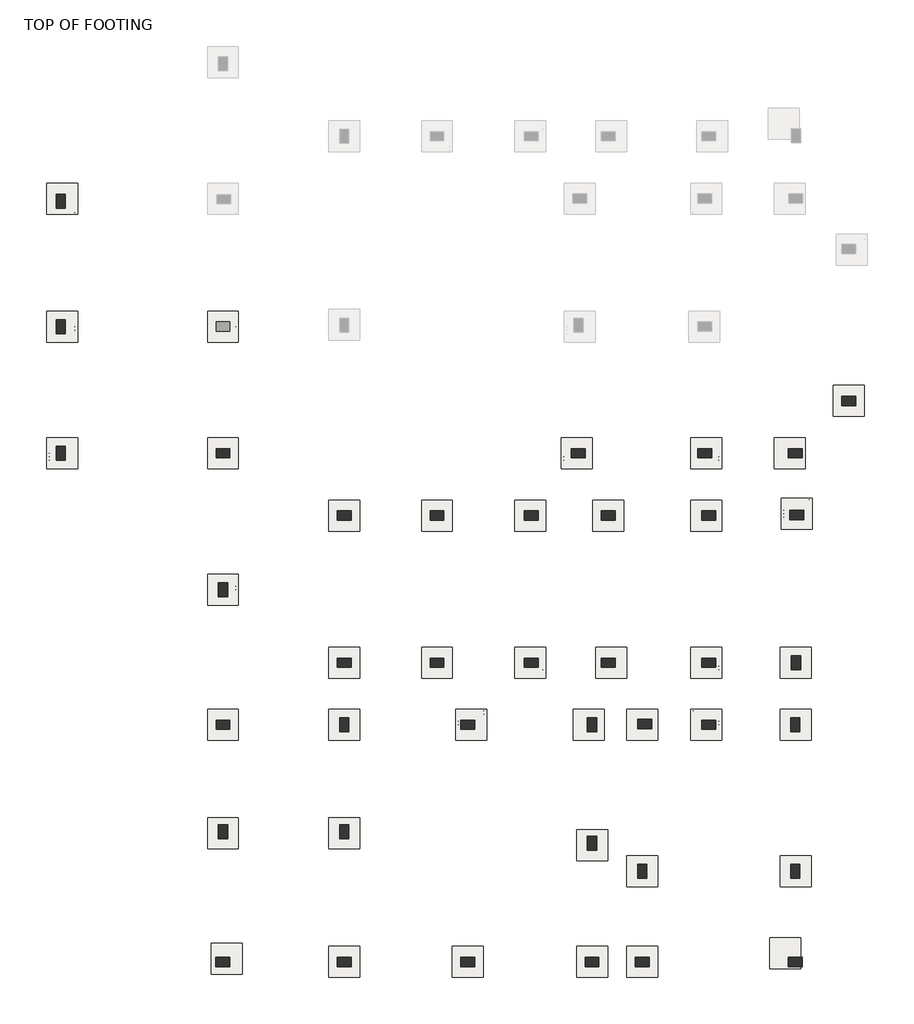
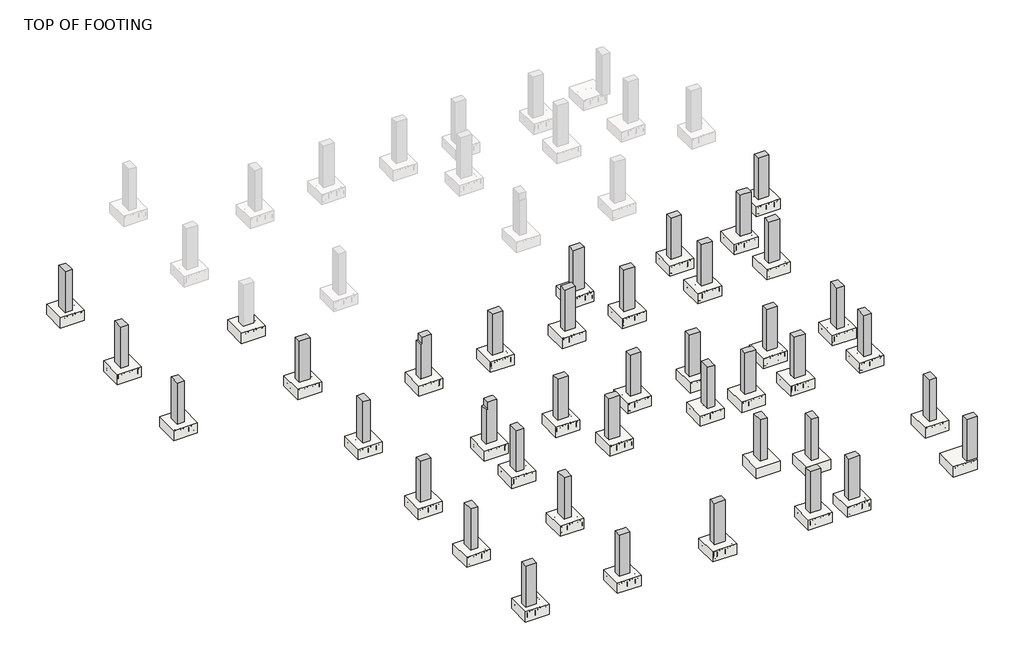
# One storey, part 1 of 20: 40 slabs, 39 columns.
"""IFC4 building model written with IfcOpenShell, lengths in millimetres."""

from ifc_helpers import new_model, si_unit, origin, place, context, project, spatial, faceted_brep, transform, mapped, element, save
from components import m_footing_rectangular_4c97ae35

model = new_model("IFC4")

# Units and contexts
model_context = context("Model", 3, world=origin())
ifc_project = project(units=[si_unit("LENGTHUNIT", "METRE", prefix="MILLI")], contexts=[model_context])

# Site, building, storey
site = spatial("IfcSite", under=ifc_project)
building = spatial("IfcBuilding", under=site)
storey = spatial("IfcBuildingStorey", under=building, Name="TOP OF FOOTING", Elevation=-1828.8)

# Columns
placement = place(None, origin())
element("IfcColumn", 1, ObjectType="M_Concrete-Rectangular-Column : 300 x 450mm", at=placement, inside=storey, context=model_context, shape_type="Brep", body=[
    faceted_brep([(-10828.8105653, 5382.6057249, -1828.8), (-10828.8105653, 4932.6057249, -1828.8), (-11128.8105653, 4932.6057249, -1828.8), (-11128.8105653, 5382.6057249, -1828.8), (-10828.8105653, 5382.6057249, 0.0), (-10828.8105653, 5067.6057249, 0.0), (-10828.8105653, 4932.6057249, 0.0), (-11128.8105653, 4932.6057249, 0.0), (-11128.8105653, 5382.6057249, 0.0)], [[[0, 1, 2, 3]], [[4, 5, 6, 1, 0]], [[6, 7, 2, 1]], [[7, 8, 3, 2]], [[8, 4, 0, 3]], [[4, 8, 7, 6, 5]]]),
])
element("IfcColumn", 2, ObjectType="M_Concrete-Rectangular-Column : 300 x 450mm", at=placement, inside=storey, context=model_context, shape_type="Brep", body=[
    faceted_brep([(-11128.8105653, 876.1713929, -1828.8), (-11128.8105653, 1326.1713929, -1828.8), (-10828.8105653, 1326.1713929, -1828.8), (-10828.8105653, 876.1713929, -1828.8), (-11128.8105653, 876.1713929, 0.0), (-11128.8105653, 1326.1713929, 0.0), (-10828.8105653, 1326.1713929, 0.0), (-10828.8105653, 1251.1713929, 0.0), (-10828.8105653, 951.1713929, 0.0), (-10828.8105653, 876.1713929, 0.0)], [[[0, 1, 2, 3]], [[4, 5, 1, 0]], [[5, 6, 2, 1]], [[6, 7, 8, 9, 3, 2]], [[9, 4, 0, 3]], [[4, 9, 8, 7, 6, 5]]]),
])
element("IfcColumn", 3, ObjectType="M_Concrete-Rectangular-Column : 300 x 450mm", at=placement, inside=storey, context=model_context, shape_type="Brep", body=[
    faceted_brep([(14244.1163908, -1148.8286071, -1828.8), (14694.1163908, -1148.8286071, -1828.8), (14694.1163908, -1448.8286071, -1828.8), (14244.1163908, -1448.8286071, -1828.8), (14244.1163908, -1148.8286071, -300.0), (14244.1163908, -1148.8286071, 0.0), (14319.1163908, -1148.8286071, 0.0), (14694.1163908, -1148.8286071, 0.0), (14694.1163908, -1448.8286071, 0.0), (14244.1163908, -1448.8286071, 0.0)], [[[0, 1, 2, 3]], [[1, 0, 4, 5, 6, 7]], [[2, 1, 7, 8]], [[3, 2, 8, 9]], [[0, 3, 9, 5, 4]], [[8, 7, 6, 5, 9]]]),
])
element("IfcColumn", 4, ObjectType="M_Concrete-Rectangular-Column : 300 x 450mm", at=placement, inside=storey, context=model_context, shape_type="Brep", body=[
    faceted_brep([(12524.1163908, -2839.4535766, -1828.8), (12974.1163908, -2839.4535766, -1828.8), (12974.1163908, -3139.4535766, -1828.8), (12524.1163908, -3139.4535766, -1828.8), (12524.1163908, -2839.4535766, -300.0), (12524.1163908, -2839.4535766, 0.0), (12599.1163908, -2839.4535766, 0.0), (12974.1163908, -2839.4535766, 0.0), (12974.1163908, -3139.4535766, 0.0), (12619.1163908, -3139.4535766, 0.0), (12524.1163908, -3139.4535766, 0.0), (12524.1163908, -3139.4535766, -300.0)], [[[0, 1, 2, 3]], [[1, 0, 4, 5, 6, 7]], [[2, 1, 7, 8]], [[3, 2, 8, 9, 10, 11]], [[0, 3, 11, 10, 5, 4]], [[8, 7, 6, 5, 10, 9]]]),
])
element("IfcColumn", 5, ObjectType="M_Concrete-Rectangular-Column : 300 x 450mm", at=placement, inside=storey, context=model_context, shape_type="Brep", body=[
    faceted_brep([(9601.8679014, -2839.4535766, -1828.8), (10051.8679014, -2839.4535766, -1828.8), (10051.8679014, -3139.4535766, -1828.8), (9601.8679014, -3139.4535766, -1828.8), (9601.8679014, -2839.4535766, -300.0), (9601.8679014, -2839.4535766, 0.0), (10051.8679014, -2839.4535766, 0.0), (10051.8679014, -2839.4535766, -300.0), (10051.8679014, -3139.4535766, 0.0), (10051.8679014, -3139.4535766, -300.0), (9601.8679014, -3139.4535766, 0.0), (9601.8679014, -3139.4535766, -300.0)], [[[0, 1, 2, 3]], [[1, 0, 4, 5, 6, 7]], [[2, 1, 7, 6, 8, 9]], [[3, 2, 9, 8, 10, 11]], [[0, 3, 11, 10, 5, 4]], [[6, 5, 10, 8]]]),
])
element("IfcColumn", 6, ObjectType="M_Concrete-Rectangular-Column : 300 x 450mm", at=placement, inside=storey, context=model_context, shape_type="Brep", body=[
    faceted_brep([(5517.5248054, -2839.4535766, -1828.8), (5967.5248054, -2839.4535766, -1828.8), (5967.5248054, -3139.4535766, -1828.8), (5517.5248054, -3139.4535766, -1828.8), (5517.5248054, -2839.4535766, -300.0), (5517.5248054, -2839.4535766, 0.0), (5967.5248054, -2839.4535766, 0.0), (5967.5248054, -2839.4535766, -300.0), (5967.5248054, -3139.4535766, 0.0), (5967.5248054, -3139.4535766, -300.0), (5517.5248054, -3139.4535766, 0.0), (5517.5248054, -3139.4535766, -300.0)], [[[0, 1, 2, 3]], [[1, 0, 4, 5, 6, 7]], [[2, 1, 7, 6, 8, 9]], [[3, 2, 9, 8, 10, 11]], [[0, 3, 11, 10, 5, 4]], [[6, 5, 10, 8]]]),
])
element("IfcColumn", 7, ObjectType="M_Concrete-Rectangular-Column : 300 x 450mm", at=placement, inside=storey, context=model_context, shape_type="Brep", body=[
    faceted_brep([(-11128.8105653, -3214.4535766, -1828.8), (-11128.8105653, -2764.4535766, -1828.8), (-10828.8105653, -2764.4535766, -1828.8), (-10828.8105653, -3214.4535766, -1828.8), (-11128.8105653, -3214.4535766, 0.0), (-11128.8105653, -2764.4535766, 0.0), (-10828.8105653, -2764.4535766, 0.0), (-10828.8105653, -2839.4535766, 0.0), (-10828.8105653, -3214.4535766, 0.0)], [[[0, 1, 2, 3]], [[4, 5, 1, 0]], [[5, 6, 2, 1]], [[6, 7, 8, 3, 2]], [[8, 4, 0, 3]], [[4, 8, 7, 6, 5]]]),
])
element("IfcColumn", 8, ObjectType="M_Concrete-Rectangular-Column : 300 x 450mm", at=placement, inside=storey, context=model_context, shape_type="Brep", body=[
    faceted_brep([(-5513.8105653, -3139.4535766, -1828.8), (-5963.8105653, -3139.4535766, -1828.8), (-5963.8105653, -2839.4535766, -1828.8), (-5513.8105653, -2839.4535766, -1828.8), (-5513.8105653, -3139.4535766, -300.0), (-5513.8105653, -3139.4535766, 0.0), (-5588.8105653, -3139.4535766, 0.0), (-5963.8105653, -3139.4535766, 0.0), (-5963.8105653, -2839.4535766, 0.0), (-5963.8105653, -2839.4535766, -300.0), (-5513.8105653, -2839.4535766, 0.0), (-5513.8105653, -2839.4535766, -300.0)], [[[0, 1, 2, 3]], [[1, 0, 4, 5, 6, 7]], [[2, 1, 7, 8, 9]], [[3, 2, 9, 8, 10, 11]], [[0, 3, 11, 10, 5, 4]], [[8, 7, 6, 5, 10]]]),
])
element("IfcColumn", 9, ObjectType="M_Concrete-Rectangular-Column : 300 x 450mm", at=placement, inside=storey, context=model_context, shape_type="Brep", body=[
    faceted_brep([(-1596.7865686, -5151.6229916, -1828.8), (-2046.7865686, -5151.6229916, -1828.8), (-2046.7865686, -4851.6229916, -1828.8), (-1596.7865686, -4851.6229916, -1828.8), (-1596.7865686, -5151.6229916, -300.0), (-1596.7865686, -5151.6229916, 0.0), (-1671.7865686, -5151.6229916, 0.0), (-1971.7865686, -5151.6229916, 0.0), (-1971.7865686, -5151.6229916, -300.0), (-2046.7865686, -5151.6229916, -300.0), (-2046.7865686, -4851.6229916, -300.0), (-1971.7865686, -4851.6229916, -300.0), (-1971.7865686, -4851.6229916, 0.0), (-1671.7865686, -4851.6229916, 0.0), (-1596.7865686, -4851.6229916, 0.0), (-1596.7865686, -4851.6229916, -300.0)], [[[0, 1, 2, 3]], [[1, 0, 4, 5, 6, 7, 8, 9]], [[2, 1, 9, 10]], [[3, 2, 10, 11, 12, 13, 14, 15]], [[0, 3, 15, 14, 5, 4]], [[5, 14, 13, 12, 7, 6]], [[8, 11, 10, 9]], [[11, 8, 7, 12]]]),
])
element("IfcColumn", 10, ObjectType="M_Concrete-Rectangular-Column : 300 x 450mm", at=placement, inside=storey, context=model_context, shape_type="Brep", body=[
    faceted_brep([(1399.7296816, -5151.6229916, -1828.8), (949.7296816, -5151.6229916, -1828.8), (949.7296816, -4851.6229916, -1828.8), (1399.7296816, -4851.6229916, -1828.8), (1399.7296816, -5151.6229916, -300.0), (1399.7296816, -5151.6229916, 0.0), (949.7296816, -5151.6229916, 0.0), (949.7296816, -5151.6229916, -300.0), (949.7296816, -4851.6229916, 0.0), (949.7296816, -4851.6229916, -300.0), (1399.7296816, -4851.6229916, 0.0), (1399.7296816, -4851.6229916, -300.0)], [[[0, 1, 2, 3]], [[1, 0, 4, 5, 6, 7]], [[2, 1, 7, 6, 8, 9]], [[3, 2, 9, 8, 10, 11]], [[0, 3, 11, 10, 5, 4]], [[6, 5, 10, 8]]]),
])
element("IfcColumn", 11, ObjectType="M_Concrete-Rectangular-Column : 300 x 450mm", at=placement, inside=storey, context=model_context, shape_type="Brep", body=[
    faceted_brep([(4447.5248054, -5151.6229916, -1828.8), (3997.5248054, -5151.6229916, -1828.8), (3997.5248054, -4851.6229916, -1828.8), (4447.5248054, -4851.6229916, -1828.8), (4447.5248054, -5151.6229916, -300.0), (4447.5248054, -5151.6229916, 0.0), (3997.5248054, -5151.6229916, 0.0), (3997.5248054, -5151.6229916, -300.0), (3997.5248054, -4851.6229916, 0.0), (3997.5248054, -4851.6229916, -300.0), (4447.5248054, -4851.6229916, 0.0), (4447.5248054, -4851.6229916, -300.0)], [[[0, 1, 2, 3]], [[1, 0, 4, 5, 6, 7]], [[2, 1, 7, 6, 8, 9]], [[3, 2, 9, 8, 10, 11]], [[0, 3, 11, 10, 5, 4]], [[6, 5, 10, 8]]]),
])
element("IfcColumn", 12, ObjectType="M_Concrete-Rectangular-Column : 300 x 450mm", at=placement, inside=storey, context=model_context, shape_type="Brep", body=[
    faceted_brep([(6931.8679014, -5151.6229916, -1828.8), (6481.8679014, -5151.6229916, -1828.8), (6481.8679014, -4851.6229916, -1828.8), (6931.8679014, -4851.6229916, -1828.8), (6931.8679014, -5151.6229916, -300.0), (6931.8679014, -5151.6229916, 0.0), (6481.8679014, -5151.6229916, 0.0), (6481.8679014, -5151.6229916, -300.0), (6481.8679014, -4851.6229916, 0.0), (6931.8679014, -4851.6229916, 0.0)], [[[0, 1, 2, 3]], [[1, 0, 4, 5, 6, 7]], [[2, 1, 7, 6, 8]], [[3, 2, 8, 9]], [[0, 3, 9, 5, 4]], [[6, 5, 9, 8]]]),
])
element("IfcColumn", 13, ObjectType="M_Concrete-Rectangular-Column : 300 x 450mm", at=placement, inside=storey, context=model_context, shape_type="Brep", body=[
    faceted_brep([(10171.8679014, -5151.6229916, -1828.8), (9721.8679014, -5151.6229916, -1828.8), (9721.8679014, -4851.6229916, -1828.8), (10171.8679014, -4851.6229916, -1828.8), (10171.8679014, -5151.6229916, -300.0), (10171.8679014, -5151.6229916, 0.0), (9721.8679014, -5151.6229916, 0.0), (9721.8679014, -5151.6229916, -300.0), (9721.8679014, -4851.6229916, 0.0), (10171.8679014, -4851.6229916, 0.0)], [[[0, 1, 2, 3]], [[1, 0, 4, 5, 6, 7]], [[2, 1, 7, 6, 8]], [[3, 2, 8, 9]], [[0, 3, 9, 5, 4]], [[6, 5, 9, 8]]]),
])
element("IfcColumn", 14, ObjectType="M_Concrete-Rectangular-Column : 300 x 450mm", at=placement, inside=storey, context=model_context, shape_type="Brep", body=[
    faceted_brep([(13014.1163908, -5131.6229916, -1828.8), (12564.1163908, -5131.6229916, -1828.8), (12564.1163908, -4831.6229916, -1828.8), (13014.1163908, -4831.6229916, -1828.8), (13014.1163908, -5131.6229916, 0.0), (12564.1163908, -5131.6229916, 0.0), (12564.1163908, -4831.6229916, 0.0), (12564.1163908, -4831.6229916, -300.0), (12619.1163908, -4831.6229916, 0.0), (13014.1163908, -4831.6229916, 0.0)], [[[0, 1, 2, 3]], [[1, 0, 4, 5]], [[2, 1, 5, 6, 7]], [[3, 2, 7, 6, 8, 9]], [[0, 3, 9, 4]], [[5, 4, 9, 8, 6]]]),
])
element("IfcColumn", 15, ObjectType="M_Concrete-Rectangular-Column : 300 x 450mm", at=placement, inside=storey, context=model_context, shape_type="Brep", body=[
    faceted_brep([(-1596.7865686, -9907.1078267, -1828.8), (-2046.7865686, -9907.1078267, -1828.8), (-2046.7865686, -9607.1078267, -1828.8), (-1596.7865686, -9607.1078267, -1828.8), (-1596.7865686, -9907.1078267, -300.0), (-1596.7865686, -9907.1078267, 0.0), (-1671.7865686, -9907.1078267, 0.0), (-1971.7865686, -9907.1078267, 0.0), (-1971.7865686, -9907.1078267, -300.0), (-2046.7865686, -9907.1078267, -300.0), (-2046.7865686, -9607.1078267, -300.0), (-1971.7865686, -9607.1078267, -300.0), (-1971.7865686, -9607.1078267, 0.0), (-1671.7865686, -9607.1078267, 0.0), (-1596.7865686, -9607.1078267, 0.0), (-1596.7865686, -9607.1078267, -300.0)], [[[0, 1, 2, 3]], [[1, 0, 4, 5, 6, 7, 8, 9]], [[2, 1, 9, 10]], [[3, 2, 10, 11, 12, 13, 14, 15]], [[0, 3, 15, 14, 5, 4]], [[5, 14, 13, 12, 7, 6]], [[8, 11, 10, 9]], [[11, 8, 7, 12]]]),
])
element("IfcColumn", 16, ObjectType="M_Concrete-Rectangular-Column : 300 x 450mm", at=placement, inside=storey, context=model_context, shape_type="Brep", body=[
    faceted_brep([(1399.7296816, -9907.1078267, -1828.8), (949.7296816, -9907.1078267, -1828.8), (949.7296816, -9607.1078267, -1828.8), (1399.7296816, -9607.1078267, -1828.8), (1399.7296816, -9907.1078267, -300.0), (1399.7296816, -9907.1078267, 0.0), (949.7296816, -9907.1078267, 0.0), (949.7296816, -9907.1078267, -300.0), (949.7296816, -9607.1078267, 0.0), (949.7296816, -9607.1078267, -300.0), (1399.7296816, -9607.1078267, 0.0), (1399.7296816, -9607.1078267, -300.0)], [[[0, 1, 2, 3]], [[1, 0, 4, 5, 6, 7]], [[2, 1, 7, 6, 8, 9]], [[3, 2, 9, 8, 10, 11]], [[0, 3, 11, 10, 5, 4]], [[6, 5, 10, 8]]]),
])
element("IfcColumn", 17, ObjectType="M_Concrete-Rectangular-Column : 300 x 450mm", at=placement, inside=storey, context=model_context, shape_type="Brep", body=[
    faceted_brep([(4447.5248054, -9907.1078267, -1828.8), (3997.5248054, -9907.1078267, -1828.8), (3997.5248054, -9607.1078267, -1828.8), (4447.5248054, -9607.1078267, -1828.8), (4447.5248054, -9907.1078267, -300.0), (4447.5248054, -9907.1078267, 0.0), (3997.5248054, -9907.1078267, 0.0), (3997.5248054, -9907.1078267, -300.0), (3997.5248054, -9607.1078267, 0.0), (3997.5248054, -9607.1078267, -300.0), (4447.5248054, -9607.1078267, 0.0), (4447.5248054, -9607.1078267, -300.0)], [[[0, 1, 2, 3]], [[1, 0, 4, 5, 6, 7]], [[2, 1, 7, 6, 8, 9]], [[3, 2, 9, 8, 10, 11]], [[0, 3, 11, 10, 5, 4]], [[6, 5, 10, 8]]]),
])
element("IfcColumn", 18, ObjectType="M_Concrete-Rectangular-Column : 300 x 450mm", at=placement, inside=storey, context=model_context, shape_type="Brep", body=[
    faceted_brep([(6931.8679014, -9907.1078267, -1828.8), (6481.8679014, -9907.1078267, -1828.8), (6481.8679014, -9607.1078267, -1828.8), (6931.8679014, -9607.1078267, -1828.8), (6931.8679014, -9907.1078267, -300.0), (6931.8679014, -9907.1078267, 0.0), (6481.8679014, -9907.1078267, 0.0), (6481.8679014, -9907.1078267, -300.0), (6481.8679014, -9607.1078267, 0.0), (6481.8679014, -9607.1078267, -300.0), (6931.8679014, -9607.1078267, 0.0), (6931.8679014, -9607.1078267, -300.0)], [[[0, 1, 2, 3]], [[1, 0, 4, 5, 6, 7]], [[2, 1, 7, 6, 8, 9]], [[3, 2, 9, 8, 10, 11]], [[0, 3, 11, 10, 5, 4]], [[6, 5, 10, 8]]]),
])
element("IfcColumn", 19, ObjectType="M_Concrete-Rectangular-Column : 300 x 450mm", at=placement, inside=storey, context=model_context, shape_type="Brep", body=[
    faceted_brep([(10171.8679014, -9907.1078267, -1828.8), (9721.8679014, -9907.1078267, -1828.8), (9721.8679014, -9607.1078267, -1828.8), (10171.8679014, -9607.1078267, -1828.8), (10171.8679014, -9907.1078267, -300.0), (10171.8679014, -9907.1078267, 0.0), (9721.8679014, -9907.1078267, 0.0), (9721.8679014, -9907.1078267, -300.0), (9721.8679014, -9607.1078267, 0.0), (9721.8679014, -9607.1078267, -300.0), (10171.8679014, -9607.1078267, 0.0), (10171.8679014, -9607.1078267, -300.0)], [[[0, 1, 2, 3]], [[1, 0, 4, 5, 6, 7]], [[2, 1, 7, 6, 8, 9]], [[3, 2, 9, 8, 10, 11]], [[0, 3, 11, 10, 5, 4]], [[6, 5, 10, 8]]]),
])
element("IfcColumn", 20, ObjectType="M_Concrete-Rectangular-Column : 300 x 450mm", at=placement, inside=storey, context=model_context, shape_type="Brep", body=[
    faceted_brep([(12919.1163908, -9532.1078267, -1828.8), (12919.1163908, -9982.1078267, -1828.8), (12619.1163908, -9982.1078267, -1828.8), (12619.1163908, -9532.1078267, -1828.8), (12919.1163908, -9532.1078267, 0.0), (12919.1163908, -9982.1078267, 0.0), (12619.1163908, -9982.1078267, 0.0), (12619.1163908, -9607.1078267, 0.0), (12619.1163908, -9532.1078267, 0.0), (12619.1163908, -9532.1078267, -300.0)], [[[0, 1, 2, 3]], [[1, 0, 4, 5]], [[2, 1, 5, 6]], [[3, 2, 6, 7, 8, 9]], [[0, 3, 9, 8, 4]], [[5, 4, 8, 7, 6]]]),
])
element("IfcColumn", 21, ObjectType="M_Concrete-Rectangular-Column : 300 x 450mm", at=placement, inside=storey, context=model_context, shape_type="Brep", body=[
    faceted_brep([(12899.1163908, -11532.8970059, -1828.8), (12899.1163908, -11982.8970059, -1828.8), (12599.1163908, -11982.8970059, -1828.8), (12599.1163908, -11532.8970059, -1828.8), (12899.1163908, -11532.8970059, 0.0), (12899.1163908, -11982.8970059, 0.0), (12599.1163908, -11982.8970059, 0.0), (12599.1163908, -11982.8970059, -300.0), (12599.1163908, -11907.8970059, 0.0), (12599.1163908, -11607.8970059, 0.0), (12599.1163908, -11532.8970059, 0.0), (12599.1163908, -11532.8970059, -300.0)], [[[0, 1, 2, 3]], [[1, 0, 4, 5]], [[2, 1, 5, 6, 7]], [[3, 2, 7, 6, 8, 9, 10, 11]], [[0, 3, 11, 10, 4]], [[5, 4, 10, 9, 8, 6]]]),
])
element("IfcColumn", 22, ObjectType="M_Concrete-Rectangular-Column : 300 x 450mm", at=placement, inside=storey, context=model_context, shape_type="Brep", body=[
    faceted_brep([(9721.8679014, -11607.8970059, -1828.8), (10171.8679014, -11607.8970059, -1828.8), (10171.8679014, -11907.8970059, -1828.8), (9721.8679014, -11907.8970059, -1828.8), (9721.8679014, -11607.8970059, -300.0), (9721.8679014, -11607.8970059, 0.0), (10171.8679014, -11607.8970059, 0.0), (10171.8679014, -11607.8970059, -300.0), (10171.8679014, -11907.8970059, 0.0), (10171.8679014, -11907.8970059, -300.0), (9721.8679014, -11907.8970059, 0.0), (9721.8679014, -11907.8970059, -300.0)], [[[0, 1, 2, 3]], [[1, 0, 4, 5, 6, 7]], [[2, 1, 7, 6, 8, 9]], [[3, 2, 9, 8, 10, 11]], [[0, 3, 11, 10, 5, 4]], [[6, 5, 10, 8]]]),
])
element("IfcColumn", 23, ObjectType="M_Concrete-Rectangular-Column : 300 x 450mm", at=placement, inside=storey, context=model_context, shape_type="Brep", body=[
    faceted_brep([(7661.8679014, -11587.8970059, -1828.8), (8111.8679014, -11587.8970059, -1828.8), (8111.8679014, -11887.8970059, -1828.8), (7661.8679014, -11887.8970059, -1828.8), (7661.8679014, -11587.8970059, 0.0), (7956.8679014, -11587.8970059, 0.0), (7956.8679014, -11587.8970059, -300.0), (8111.8679014, -11587.8970059, -300.0), (8111.8679014, -11607.8970059, -300.0), (8111.8679014, -11607.8970059, 0.0), (8111.8679014, -11887.8970059, 0.0), (8111.8679014, -11887.8970059, -600.0), (7661.8679014, -11887.8970059, 0.0), (7661.8679014, -11887.8970059, -600.0), (7661.8679014, -11607.8970059, 0.0), (7956.8679014, -11607.8970059, 0.0), (7956.8679014, -11607.8970059, -300.0)], [[[0, 1, 2, 3]], [[1, 0, 4, 5, 6, 7]], [[2, 1, 7, 8, 9, 10, 11]], [[3, 2, 11, 10, 12, 13]], [[0, 3, 13, 12, 14, 4]], [[12, 10, 9, 15, 5, 4, 14]], [[6, 16, 8, 7]], [[16, 15, 9, 8]], [[15, 16, 6, 5]]]),
])
element("IfcColumn", 24, ObjectType="M_Concrete-Rectangular-Column : 300 x 450mm", at=placement, inside=storey, context=model_context, shape_type="Brep", body=[
    faceted_brep([(6332.5248054, -11532.8970059, -1828.8), (6332.5248054, -11982.8970059, -1828.8), (6032.5248054, -11982.8970059, -1828.8), (6032.5248054, -11532.8970059, -1828.8), (6332.5248054, -11532.8970059, -300.0), (6332.5248054, -11532.8970059, 0.0), (6332.5248054, -11607.8970059, 0.0), (6332.5248054, -11907.8970059, 0.0), (6332.5248054, -11982.8970059, 0.0), (6332.5248054, -11982.8970059, -300.0), (6032.5248054, -11982.8970059, 0.0), (6032.5248054, -11982.8970059, -300.0), (6032.5248054, -11907.8970059, 0.0), (6032.5248054, -11607.8970059, 0.0), (6032.5248054, -11532.8970059, 0.0), (6032.5248054, -11532.8970059, -300.0)], [[[0, 1, 2, 3]], [[1, 0, 4, 5, 6, 7, 8, 9]], [[2, 1, 9, 8, 10, 11]], [[3, 2, 11, 10, 12, 13, 14, 15]], [[0, 3, 15, 14, 5, 4]], [[10, 8, 7, 6, 5, 14, 13, 12]]]),
])
element("IfcColumn", 25, ObjectType="M_Concrete-Rectangular-Column : 300 x 450mm", at=placement, inside=storey, context=model_context, shape_type="Brep", body=[
    faceted_brep([(1949.7296816, -11607.8970059, -1828.8), (2399.7296816, -11607.8970059, -1828.8), (2399.7296816, -11907.8970059, -1828.8), (1949.7296816, -11907.8970059, -1828.8), (1949.7296816, -11607.8970059, -300.0), (1949.7296816, -11607.8970059, 0.0), (2024.7296816, -11607.8970059, 0.0), (2324.7296816, -11607.8970059, 0.0), (2399.7296816, -11607.8970059, 0.0), (2399.7296816, -11607.8970059, -300.0), (2399.7296816, -11907.8970059, 0.0), (2399.7296816, -11907.8970059, -300.0), (2324.7296816, -11907.8970059, 0.0), (2024.7296816, -11907.8970059, 0.0), (1949.7296816, -11907.8970059, 0.0), (1949.7296816, -11907.8970059, -300.0)], [[[0, 1, 2, 3]], [[1, 0, 4, 5, 6, 7, 8, 9]], [[2, 1, 9, 8, 10, 11]], [[3, 2, 11, 10, 12, 13, 14, 15]], [[0, 3, 15, 14, 5, 4]], [[10, 8, 7, 6, 5, 14, 13, 12]]]),
])
element("IfcColumn", 26, ObjectType="M_Concrete-Rectangular-Column : 300 x 450mm", at=placement, inside=storey, context=model_context, shape_type="Brep", body=[
    faceted_brep([(-1971.7865686, -11982.8970059, -1828.8), (-1971.7865686, -11532.8970059, -1828.8), (-1671.7865686, -11532.8970059, -1828.8), (-1671.7865686, -11982.8970059, -1828.8), (-1971.7865686, -11982.8970059, -300.0), (-1971.7865686, -11982.8970059, 0.0), (-1971.7865686, -11907.8970059, 0.0), (-1971.7865686, -11607.8970059, 0.0), (-1971.7865686, -11532.8970059, 0.0), (-1971.7865686, -11532.8970059, -300.0), (-1671.7865686, -11532.8970059, 0.0), (-1671.7865686, -11532.8970059, -300.0), (-1671.7865686, -11607.8970059, 0.0), (-1671.7865686, -11907.8970059, 0.0), (-1671.7865686, -11982.8970059, 0.0), (-1671.7865686, -11982.8970059, -300.0)], [[[0, 1, 2, 3]], [[1, 0, 4, 5, 6, 7, 8, 9]], [[2, 1, 9, 8, 10, 11]], [[3, 2, 11, 10, 12, 13, 14, 15]], [[0, 3, 15, 14, 5, 4]], [[10, 8, 7, 6, 5, 14, 13, 12]]]),
])
element("IfcColumn", 27, ObjectType="M_Concrete-Rectangular-Column : 300 x 450mm", at=placement, inside=storey, context=model_context, shape_type="Brep", body=[
    faceted_brep([(-5513.8105653, -11907.8970059, -1828.8), (-5963.8105653, -11907.8970059, -1828.8), (-5963.8105653, -11607.8970059, -1828.8), (-5513.8105653, -11607.8970059, -1828.8), (-5513.8105653, -11907.8970059, -300.0), (-5513.8105653, -11907.8970059, 0.0), (-5588.8105653, -11907.8970059, 0.0), (-5963.8105653, -11907.8970059, 0.0), (-5963.8105653, -11607.8970059, 0.0), (-5588.8105653, -11607.8970059, 0.0), (-5513.8105653, -11607.8970059, 0.0), (-5513.8105653, -11607.8970059, -300.0)], [[[0, 1, 2, 3]], [[1, 0, 4, 5, 6, 7]], [[2, 1, 7, 8]], [[3, 2, 8, 9, 10, 11]], [[0, 3, 11, 10, 5, 4]], [[8, 7, 6, 5, 10, 9]]]),
])
element("IfcColumn", 28, ObjectType="M_Concrete-Rectangular-Column : 300 x 450mm", at=placement, inside=storey, context=model_context, shape_type="Brep", body=[
    faceted_brep([(-5588.8105653, -14991.2517597, -1828.8), (-5588.8105653, -15441.2517597, -1828.8), (-5888.8105653, -15441.2517597, -1828.8), (-5888.8105653, -14991.2517597, -1828.8), (-5588.8105653, -14991.2517597, -300.0), (-5588.8105653, -14991.2517597, 0.0), (-5588.8105653, -15441.2517597, 0.0), (-5588.8105653, -15441.2517597, -300.0), (-5888.8105653, -15441.2517597, 0.0), (-5888.8105653, -14991.2517597, 0.0)], [[[0, 1, 2, 3]], [[1, 0, 4, 5, 6, 7]], [[2, 1, 7, 6, 8]], [[3, 2, 8, 9]], [[0, 3, 9, 5, 4]], [[6, 5, 9, 8]]]),
])
element("IfcColumn", 29, ObjectType="M_Concrete-Rectangular-Column : 300 x 450mm", at=placement, inside=storey, context=model_context, shape_type="Brep", body=[
    faceted_brep([(-1671.7865686, -14991.2517597, -1828.8), (-1671.7865686, -15441.2517597, -1828.8), (-1971.7865686, -15441.2517597, -1828.8), (-1971.7865686, -14991.2517597, -1828.8), (-1671.7865686, -14991.2517597, -300.0), (-1671.7865686, -14991.2517597, 0.0), (-1671.7865686, -15441.2517597, 0.0), (-1671.7865686, -15441.2517597, -300.0), (-1971.7865686, -15441.2517597, 0.0), (-1971.7865686, -15441.2517597, -300.0), (-1971.7865686, -14991.2517597, 0.0), (-1971.7865686, -14991.2517597, -300.0)], [[[0, 1, 2, 3]], [[1, 0, 4, 5, 6, 7]], [[2, 1, 7, 6, 8, 9]], [[3, 2, 9, 8, 10, 11]], [[0, 3, 11, 10, 5, 4]], [[6, 5, 10, 8]]]),
])
element("IfcColumn", 30, ObjectType="M_Concrete-Rectangular-Column : 300 x 450mm", at=placement, inside=storey, context=model_context, shape_type="Brep", body=[
    faceted_brep([(-2046.7865686, -19272.5304373, -1828.8), (-1596.7865686, -19272.5304373, -1828.8), (-1596.7865686, -19572.5304373, -1828.8), (-2046.7865686, -19572.5304373, -1828.8), (-2046.7865686, -19272.5304373, 0.0), (-1971.7865686, -19272.5304373, 0.0), (-1671.7865686, -19272.5304373, 0.0), (-1596.7865686, -19272.5304373, 0.0), (-1596.7865686, -19572.5304373, 0.0), (-2046.7865686, -19572.5304373, 0.0)], [[[0, 1, 2, 3]], [[4, 5, 6, 7, 1, 0]], [[7, 8, 2, 1]], [[8, 9, 3, 2]], [[9, 4, 0, 3]], [[4, 9, 8, 7, 6, 5]]]),
])
element("IfcColumn", 31, ObjectType="M_Concrete-Rectangular-Column : 300 x 450mm", at=placement, inside=storey, context=model_context, shape_type="Brep", body=[
    faceted_brep([(1949.7296816, -19272.5304373, -1828.8), (2399.7296816, -19272.5304373, -1828.8), (2399.7296816, -19572.5304373, -1828.8), (1949.7296816, -19572.5304373, -1828.8), (1949.7296816, -19272.5304373, 0.0), (2024.7296816, -19272.5304373, 0.0), (2324.7296816, -19272.5304373, 0.0), (2399.7296816, -19272.5304373, 0.0), (2399.7296816, -19572.5304373, 0.0), (1949.7296816, -19572.5304373, 0.0)], [[[0, 1, 2, 3]], [[4, 5, 6, 7, 1, 0]], [[7, 8, 2, 1]], [[8, 9, 3, 2]], [[9, 4, 0, 3]], [[4, 9, 8, 7, 6, 5]]]),
])
element("IfcColumn", 32, ObjectType="M_Concrete-Rectangular-Column : 300 x 450mm", at=placement, inside=storey, context=model_context, shape_type="Brep", body=[
    faceted_brep([(5957.5248054, -19272.5304373, -1828.8), (6407.5248054, -19272.5304373, -1828.8), (6407.5248054, -19572.5304373, -1828.8), (5957.5248054, -19572.5304373, -1828.8), (5957.5248054, -19272.5304373, 0.0), (6032.5248054, -19272.5304373, 0.0), (6332.5248054, -19272.5304373, 0.0), (6407.5248054, -19272.5304373, 0.0), (6407.5248054, -19572.5304373, 0.0), (5957.5248054, -19572.5304373, 0.0)], [[[0, 1, 2, 3]], [[4, 5, 6, 7, 1, 0]], [[7, 8, 2, 1]], [[8, 9, 3, 2]], [[9, 4, 0, 3]], [[4, 9, 8, 7, 6, 5]]]),
])
element("IfcColumn", 33, ObjectType="M_Concrete-Rectangular-Column : 300 x 450mm", at=placement, inside=storey, context=model_context, shape_type="Brep", body=[
    faceted_brep([(7581.8679014, -19272.5304373, -1828.8), (8031.8679014, -19272.5304373, -1828.8), (8031.8679014, -19572.5304373, -1828.8), (7581.8679014, -19572.5304373, -1828.8), (7581.8679014, -19272.5304373, 0.0), (7656.8679014, -19272.5304373, 0.0), (7956.8679014, -19272.5304373, 0.0), (8031.8679014, -19272.5304373, 0.0), (8031.8679014, -19572.5304373, 0.0), (7581.8679014, -19572.5304373, 0.0)], [[[0, 1, 2, 3]], [[4, 5, 6, 7, 1, 0]], [[7, 8, 2, 1]], [[8, 9, 3, 2]], [[9, 4, 0, 3]], [[4, 9, 8, 7, 6, 5]]]),
])
element("IfcColumn", 34, ObjectType="M_Concrete-Rectangular-Column : 300 x 450mm", at=placement, inside=storey, context=model_context, shape_type="Brep", body=[
    faceted_brep([(12599.1163908, -16719.1579597, -1828.8), (12599.1163908, -16269.1579597, -1828.8), (12899.1163908, -16269.1579597, -1828.8), (12899.1163908, -16719.1579597, -1828.8), (12599.1163908, -16719.1579597, -300.0), (12599.1163908, -16719.1579597, 0.0), (12599.1163908, -16644.1579597, 0.0), (12599.1163908, -16344.1579597, 0.0), (12599.1163908, -16269.1579597, 0.0), (12599.1163908, -16269.1579597, -300.0), (12899.1163908, -16269.1579597, 0.0), (12899.1163908, -16719.1579597, 0.0)], [[[0, 1, 2, 3]], [[1, 0, 4, 5, 6, 7, 8, 9]], [[2, 1, 9, 8, 10]], [[3, 2, 10, 11]], [[0, 3, 11, 5, 4]], [[10, 8, 7, 6, 5, 11]]]),
])
element("IfcColumn", 35, ObjectType="M_Concrete-Rectangular-Column : 300 x 450mm", at=placement, inside=storey, context=model_context, shape_type="Brep", body=[
    faceted_brep([(7656.8679014, -16719.1579597, -1828.8), (7656.8679014, -16269.1579597, -1828.8), (7956.8679014, -16269.1579597, -1828.8), (7956.8679014, -16719.1579597, -1828.8), (7656.8679014, -16719.1579597, -300.0), (7656.8679014, -16719.1579597, 0.0), (7656.8679014, -16269.1579597, 0.0), (7656.8679014, -16269.1579597, -300.0), (7956.8679014, -16269.1579597, 0.0), (7956.8679014, -16269.1579597, -300.0), (7956.8679014, -16344.1579597, 0.0), (7956.8679014, -16644.1579597, 0.0), (7956.8679014, -16719.1579597, 0.0), (7956.8679014, -16719.1579597, -300.0)], [[[0, 1, 2, 3]], [[1, 0, 4, 5, 6, 7]], [[2, 1, 7, 6, 8, 9]], [[3, 2, 9, 8, 10, 11, 12, 13]], [[0, 3, 13, 12, 5, 4]], [[6, 5, 12, 11, 10, 8]]]),
])
element("IfcColumn", 36, ObjectType="M_Concrete-Rectangular-Column : 300 x 450mm", at=placement, inside=storey, context=model_context, shape_type="Brep", body=[
    faceted_brep([(6032.5248054, -15819.1579597, -1828.8), (6032.5248054, -15369.1579597, -1828.8), (6332.5248054, -15369.1579597, -1828.8), (6332.5248054, -15819.1579597, -1828.8), (6032.5248054, -15819.1579597, -300.0), (6032.5248054, -15819.1579597, 0.0), (6032.5248054, -15369.1579597, 0.0), (6032.5248054, -15369.1579597, -300.0), (6332.5248054, -15369.1579597, 0.0), (6332.5248054, -15369.1579597, -300.0), (6332.5248054, -15819.1579597, 0.0), (6332.5248054, -15819.1579597, -300.0)], [[[0, 1, 2, 3]], [[1, 0, 4, 5, 6, 7]], [[2, 1, 7, 6, 8, 9]], [[3, 2, 9, 8, 10, 11]], [[0, 3, 11, 10, 5, 4]], [[6, 5, 10, 8]]]),
])
element("IfcColumn", 37, ObjectType="M_Concrete-Rectangular-Column : 300 x 450mm", at=placement, inside=storey, context=model_context, shape_type="Brep", body=[
    faceted_brep([(12974.1163908, -19572.5304373, -1828.8), (12524.1163908, -19572.5304373, -1828.8), (12524.1163908, -19272.5304373, -1828.8), (12974.1163908, -19272.5304373, -1828.8), (12974.1163908, -19572.5304373, 0.0), (12524.1163908, -19572.5304373, 0.0), (12524.1163908, -19272.5304373, 0.0), (12599.1163908, -19272.5304373, 0.0), (12974.1163908, -19272.5304373, 0.0)], [[[0, 1, 2, 3]], [[4, 5, 1, 0]], [[5, 6, 2, 1]], [[6, 7, 8, 3, 2]], [[8, 4, 0, 3]], [[4, 8, 7, 6, 5]]]),
])
element("IfcColumn", 38, ObjectType="M_Concrete-Rectangular-Column : 300 x 450mm", at=placement, inside=storey, context=model_context, shape_type="Brep", body=[
    faceted_brep([(-5516.7865686, -19572.5304373, -1828.8), (-5966.7865686, -19572.5304373, -1828.8), (-5966.7865686, -19272.5304373, -1828.8), (-5516.7865686, -19272.5304373, -1828.8), (-5516.7865686, -19572.5304373, 0.0), (-5966.7865686, -19572.5304373, 0.0), (-5966.7865686, -19272.5304373, 0.0), (-5588.8105653, -19272.5304373, 0.0), (-5516.7865686, -19272.5304373, 0.0)], [[[0, 1, 2, 3]], [[4, 5, 1, 0]], [[5, 6, 2, 1]], [[6, 7, 8, 3, 2]], [[8, 4, 0, 3]], [[4, 8, 7, 6, 5]]]),
])
element("IfcColumn", 39, ObjectType="M_Concrete-Rectangular-Column : 300 x 450mm", at=placement, inside=storey, context=model_context, shape_type="Brep", body=[
    faceted_brep([(-5588.8105653, -7169.0760584, -1828.8), (-5588.8105653, -7619.0760584, -1828.8), (-5888.8105653, -7619.0760584, -1828.8), (-5888.8105653, -7169.0760584, -1828.8), (-5588.8105653, -7169.0760584, -300.0), (-5588.8105653, -7169.0760584, 0.0), (-5588.8105653, -7619.0760584, 0.0), (-5588.8105653, -7619.0760584, -300.0), (-5888.8105653, -7619.0760584, 0.0), (-5888.8105653, -7169.0760584, 0.0)], [[[0, 1, 2, 3]], [[1, 0, 4, 5, 6, 7]], [[2, 1, 7, 6, 8]], [[3, 2, 8, 9]], [[0, 3, 9, 5, 4]], [[6, 5, 9, 8]]]),
])

# Slabs
m_footing_rectangular_shape = m_footing_rectangular_4c97ae35(model_context)
element("IfcSlab", 40, ObjectType="M_Footing-Rectangular", at=placement, inside=storey, context=model_context, shape_type="MappedRepresentation", body=[
    mapped(m_footing_rectangular_shape, transform((-10938.8105653, 5237.6057249, -1828.8), x_axis=(1.0, 0.0, 0.0), y_axis=(0.0, 1.0, 0.0), z_axis=(0.0, 0.0, 1.0))),
])
element("IfcSlab", 41, ObjectType="M_Footing-Rectangular", at=placement, inside=storey, context=model_context, shape_type="MappedRepresentation", body=[
    mapped(m_footing_rectangular_shape, transform((-10938.8105653, 1101.1713929, -1828.8), x_axis=(1.0, 0.0, 0.0), y_axis=(0.0, 1.0, 0.0), z_axis=(0.0, 0.0, 1.0))),
])
element("IfcSlab", 42, ObjectType="M_Footing-Rectangular", at=placement, inside=storey, context=model_context, shape_type="MappedRepresentation", body=[
    mapped(m_footing_rectangular_shape, transform((-5738.8105653, 1101.1713929, -1828.8), x_axis=(1.0, 0.0, 0.0), y_axis=(0.0, 1.0, 0.0), z_axis=(0.0, 0.0, 1.0))),
])
element("IfcSlab", 43, ObjectType="M_Footing-Rectangular", at=placement, inside=storey, context=model_context, shape_type="MappedRepresentation", body=[
    mapped(m_footing_rectangular_shape, transform((14469.1163908, -1298.8286071, -1828.8), x_axis=(1.0, 0.0, 0.0), y_axis=(0.0, 1.0, 0.0), z_axis=(0.0, 0.0, 1.0))),
])
element("IfcSlab", 44, ObjectType="M_Footing-Rectangular", at=placement, inside=storey, context=model_context, shape_type="MappedRepresentation", body=[
    mapped(m_footing_rectangular_shape, transform((12569.1163908, -2989.4535766, -1828.8), x_axis=(1.0, 0.0, 0.0), y_axis=(0.0, 1.0, 0.0), z_axis=(0.0, 0.0, 1.0))),
])
element("IfcSlab", 45, ObjectType="M_Footing-Rectangular", at=placement, inside=storey, context=model_context, shape_type="MappedRepresentation", body=[
    mapped(m_footing_rectangular_shape, transform((9869.1163908, -2989.4535766, -1828.8), x_axis=(1.0, 0.0, 0.0), y_axis=(0.0, 1.0, 0.0), z_axis=(0.0, 0.0, 1.0))),
])
element("IfcSlab", 46, ObjectType="M_Footing-Rectangular", at=placement, inside=storey, context=model_context, shape_type="MappedRepresentation", body=[
    mapped(m_footing_rectangular_shape, transform((5682.5248054, -2989.4535766, -1828.8), x_axis=(1.0, 0.0, 0.0), y_axis=(0.0, 1.0, 0.0), z_axis=(0.0, 0.0, 1.0))),
])
element("IfcSlab", 47, ObjectType="M_Footing-Rectangular", at=placement, inside=storey, context=model_context, shape_type="MappedRepresentation", body=[
    mapped(m_footing_rectangular_shape, transform((-5738.8105653, -2989.4535766, -1828.8), x_axis=(1.0, 0.0, 0.0), y_axis=(0.0, 1.0, 0.0), z_axis=(0.0, 0.0, 1.0))),
])
element("IfcSlab", 48, ObjectType="M_Footing-Rectangular", at=placement, inside=storey, context=model_context, shape_type="MappedRepresentation", body=[
    mapped(m_footing_rectangular_shape, transform((-10938.8105653, -2989.4535766, -1828.8), x_axis=(1.0, 0.0, 0.0), y_axis=(0.0, 1.0, 0.0), z_axis=(0.0, 0.0, 1.0))),
])
element("IfcSlab", 49, ObjectType="M_Footing-Rectangular", at=placement, inside=storey, context=model_context, shape_type="MappedRepresentation", body=[
    mapped(m_footing_rectangular_shape, transform((-1821.7865686, -5001.6229916, -1828.8), x_axis=(1.0, 0.0, 0.0), y_axis=(0.0, 1.0, 0.0), z_axis=(0.0, 0.0, 1.0))),
])
element("IfcSlab", 50, ObjectType="M_Footing-Rectangular", at=placement, inside=storey, context=model_context, shape_type="MappedRepresentation", body=[
    mapped(m_footing_rectangular_shape, transform((1174.7296816, -5001.6229916, -1828.8), x_axis=(1.0, 0.0, 0.0), y_axis=(0.0, 1.0, 0.0), z_axis=(0.0, 0.0, 1.0))),
])
element("IfcSlab", 51, ObjectType="M_Footing-Rectangular", at=placement, inside=storey, context=model_context, shape_type="MappedRepresentation", body=[
    mapped(m_footing_rectangular_shape, transform((4182.5248054, -5001.6229916, -1828.8), x_axis=(1.0, 0.0, 0.0), y_axis=(0.0, 1.0, 0.0), z_axis=(0.0, 0.0, 1.0))),
])
element("IfcSlab", 52, ObjectType="M_Footing-Rectangular", at=placement, inside=storey, context=model_context, shape_type="MappedRepresentation", body=[
    mapped(m_footing_rectangular_shape, transform((6706.8679014, -5001.6229916, -1828.8), x_axis=(1.0, 0.0, 0.0), y_axis=(0.0, 1.0, 0.0), z_axis=(0.0, 0.0, 1.0))),
])
element("IfcSlab", 53, ObjectType="M_Footing-Rectangular", at=placement, inside=storey, context=model_context, shape_type="MappedRepresentation", body=[
    mapped(m_footing_rectangular_shape, transform((9869.1163908, -5001.6229916, -1828.8), x_axis=(1.0, 0.0, 0.0), y_axis=(0.0, 1.0, 0.0), z_axis=(0.0, 0.0, 1.0))),
])
element("IfcSlab", 54, ObjectType="M_Footing-Rectangular", at=placement, inside=storey, context=model_context, shape_type="MappedRepresentation", body=[
    mapped(m_footing_rectangular_shape, transform((12789.1163908, -4941.6229916, -1828.8), x_axis=(1.0, 0.0, 0.0), y_axis=(0.0, 1.0, 0.0), z_axis=(0.0, 0.0, 1.0))),
])
element("IfcSlab", 55, ObjectType="M_Footing-Rectangular", at=placement, inside=storey, context=model_context, shape_type="MappedRepresentation", body=[
    mapped(m_footing_rectangular_shape, transform((12769.1163908, -9757.1078267, -1828.8), x_axis=(1.0, 0.0, 0.0), y_axis=(0.0, 1.0, 0.0), z_axis=(0.0, 0.0, 1.0))),
])
element("IfcSlab", 56, ObjectType="M_Footing-Rectangular", at=placement, inside=storey, context=model_context, shape_type="MappedRepresentation", body=[
    mapped(m_footing_rectangular_shape, transform((9869.1163908, -9757.1078267, -1828.8), x_axis=(1.0, 0.0, 0.0), y_axis=(0.0, 1.0, 0.0), z_axis=(0.0, 0.0, 1.0))),
])
element("IfcSlab", 57, ObjectType="M_Footing-Rectangular", at=placement, inside=storey, context=model_context, shape_type="MappedRepresentation", body=[
    mapped(m_footing_rectangular_shape, transform((6806.8679014, -9757.1078267, -1828.8), x_axis=(1.0, 0.0, 0.0), y_axis=(0.0, 1.0, 0.0), z_axis=(0.0, 0.0, 1.0))),
])
element("IfcSlab", 58, ObjectType="M_Footing-Rectangular", at=placement, inside=storey, context=model_context, shape_type="MappedRepresentation", body=[
    mapped(m_footing_rectangular_shape, transform((4182.5248054, -9757.1078267, -1828.8), x_axis=(1.0, 0.0, 0.0), y_axis=(0.0, 1.0, 0.0), z_axis=(0.0, 0.0, 1.0))),
])
element("IfcSlab", 59, ObjectType="M_Footing-Rectangular", at=placement, inside=storey, context=model_context, shape_type="MappedRepresentation", body=[
    mapped(m_footing_rectangular_shape, transform((1174.7296816, -9757.1078267, -1828.8), x_axis=(1.0, 0.0, 0.0), y_axis=(0.0, 1.0, 0.0), z_axis=(0.0, 0.0, 1.0))),
])
element("IfcSlab", 60, ObjectType="M_Footing-Rectangular", at=placement, inside=storey, context=model_context, shape_type="MappedRepresentation", body=[
    mapped(m_footing_rectangular_shape, transform((-1821.7865686, -9757.1078267, -1828.8), x_axis=(1.0, 0.0, 0.0), y_axis=(0.0, 1.0, 0.0), z_axis=(0.0, 0.0, 1.0))),
])
element("IfcSlab", 61, ObjectType="M_Footing-Rectangular", at=placement, inside=storey, context=model_context, shape_type="MappedRepresentation", body=[
    mapped(m_footing_rectangular_shape, transform((-5738.8105653, -7401.6229916, -1828.8), x_axis=(1.0, 0.0, 0.0), y_axis=(0.0, 1.0, 0.0), z_axis=(0.0, 0.0, 1.0))),
])
element("IfcSlab", 62, ObjectType="M_Footing-Rectangular", at=placement, inside=storey, context=model_context, shape_type="MappedRepresentation", body=[
    mapped(m_footing_rectangular_shape, transform((-5738.8105653, -11757.8970059, -1828.8), x_axis=(1.0, 0.0, 0.0), y_axis=(0.0, 1.0, 0.0), z_axis=(0.0, 0.0, 1.0))),
])
element("IfcSlab", 63, ObjectType="M_Footing-Rectangular", at=placement, inside=storey, context=model_context, shape_type="MappedRepresentation", body=[
    mapped(m_footing_rectangular_shape, transform((-1821.7865686, -11757.8970059, -1828.8), x_axis=(1.0, 0.0, 0.0), y_axis=(0.0, 1.0, 0.0), z_axis=(0.0, 0.0, 1.0))),
])
element("IfcSlab", 64, ObjectType="M_Footing-Rectangular", at=placement, inside=storey, context=model_context, shape_type="MappedRepresentation", body=[
    mapped(m_footing_rectangular_shape, transform((2274.7296816, -11757.8970059, -1828.8), x_axis=(1.0, 0.0, 0.0), y_axis=(0.0, 1.0, 0.0), z_axis=(0.0, 0.0, 1.0))),
])
element("IfcSlab", 65, ObjectType="M_Footing-Rectangular", at=placement, inside=storey, context=model_context, shape_type="MappedRepresentation", body=[
    mapped(m_footing_rectangular_shape, transform((6082.5248054, -11757.8970059, -1828.8), x_axis=(1.0, 0.0, 0.0), y_axis=(0.0, 1.0, 0.0), z_axis=(0.0, 0.0, 1.0))),
])
element("IfcSlab", 66, ObjectType="M_Footing-Rectangular", at=placement, inside=storey, context=model_context, shape_type="MappedRepresentation", body=[
    mapped(m_footing_rectangular_shape, transform((7806.8679014, -11757.8970059, -1828.8), x_axis=(1.0, 0.0, 0.0), y_axis=(0.0, 1.0, 0.0), z_axis=(0.0, 0.0, 1.0))),
])
element("IfcSlab", 67, ObjectType="M_Footing-Rectangular", at=placement, inside=storey, context=model_context, shape_type="MappedRepresentation", body=[
    mapped(m_footing_rectangular_shape, transform((9869.1163908, -11757.8970059, -1828.8), x_axis=(1.0, 0.0, 0.0), y_axis=(0.0, 1.0, 0.0), z_axis=(0.0, 0.0, 1.0))),
])
element("IfcSlab", 68, ObjectType="M_Footing-Rectangular", at=placement, inside=storey, context=model_context, shape_type="MappedRepresentation", body=[
    mapped(m_footing_rectangular_shape, transform((12769.1163908, -11757.8970059, -1828.8), x_axis=(1.0, 0.0, 0.0), y_axis=(0.0, 1.0, 0.0), z_axis=(0.0, 0.0, 1.0))),
])
element("IfcSlab", 69, ObjectType="M_Footing-Rectangular", at=placement, inside=storey, context=model_context, shape_type="MappedRepresentation", body=[
    mapped(m_footing_rectangular_shape, transform((12769.1163908, -16494.1579597, -1828.8), x_axis=(1.0, 0.0, 0.0), y_axis=(0.0, 1.0, 0.0), z_axis=(0.0, 0.0, 1.0))),
])
element("IfcSlab", 70, ObjectType="M_Footing-Rectangular", at=placement, inside=storey, context=model_context, shape_type="MappedRepresentation", body=[
    mapped(m_footing_rectangular_shape, transform((7806.8679014, -16494.1579597, -1828.8), x_axis=(1.0, 0.0, 0.0), y_axis=(0.0, 1.0, 0.0), z_axis=(0.0, 0.0, 1.0))),
])
element("IfcSlab", 71, ObjectType="M_Footing-Rectangular", at=placement, inside=storey, context=model_context, shape_type="MappedRepresentation", body=[
    mapped(m_footing_rectangular_shape, transform((6182.5248054, -15657.8970059, -1828.8), x_axis=(1.0, 0.0, 0.0), y_axis=(0.0, 1.0, 0.0), z_axis=(0.0, 0.0, 1.0))),
])
element("IfcSlab", 72, ObjectType="M_Footing-Rectangular", at=placement, inside=storey, context=model_context, shape_type="MappedRepresentation", body=[
    mapped(m_footing_rectangular_shape, transform((-1821.7865686, -15257.8970059, -1828.8), x_axis=(1.0, 0.0, 0.0), y_axis=(0.0, 1.0, 0.0), z_axis=(0.0, 0.0, 1.0))),
])
element("IfcSlab", 73, ObjectType="M_Footing-Rectangular", at=placement, inside=storey, context=model_context, shape_type="MappedRepresentation", body=[
    mapped(m_footing_rectangular_shape, transform((-5738.8105653, -15257.8970059, -1828.8), x_axis=(1.0, 0.0, 0.0), y_axis=(0.0, 1.0, 0.0), z_axis=(0.0, 0.0, 1.0))),
])
element("IfcSlab", 74, ObjectType="M_Footing-Rectangular", at=placement, inside=storey, context=model_context, shape_type="MappedRepresentation", body=[
    mapped(m_footing_rectangular_shape, transform((-5621.7865686, -19322.5304373, -1828.8), x_axis=(1.0, 0.0, 0.0), y_axis=(0.0, 1.0, 0.0), z_axis=(0.0, 0.0, 1.0))),
])
element("IfcSlab", 75, ObjectType="M_Footing-Rectangular", at=placement, inside=storey, context=model_context, shape_type="MappedRepresentation", body=[
    mapped(m_footing_rectangular_shape, transform((-1821.7865686, -19422.5304373, -1828.8), x_axis=(1.0, 0.0, 0.0), y_axis=(0.0, 1.0, 0.0), z_axis=(0.0, 0.0, 1.0))),
])
element("IfcSlab", 76, ObjectType="M_Footing-Rectangular", at=placement, inside=storey, context=model_context, shape_type="MappedRepresentation", body=[
    mapped(m_footing_rectangular_shape, transform((2174.7296816, -19422.5304373, -1828.8), x_axis=(1.0, 0.0, 0.0), y_axis=(0.0, 1.0, 0.0), z_axis=(0.0, 0.0, 1.0))),
])
element("IfcSlab", 77, ObjectType="M_Footing-Rectangular", at=placement, inside=storey, context=model_context, shape_type="MappedRepresentation", body=[
    mapped(m_footing_rectangular_shape, transform((6182.5248054, -19422.5304373, -1828.8), x_axis=(1.0, 0.0, 0.0), y_axis=(0.0, 1.0, 0.0), z_axis=(0.0, 0.0, 1.0))),
])
element("IfcSlab", 78, ObjectType="M_Footing-Rectangular", at=placement, inside=storey, context=model_context, shape_type="MappedRepresentation", body=[
    mapped(m_footing_rectangular_shape, transform((7806.8679014, -19422.5304373, -1828.8), x_axis=(1.0, 0.0, 0.0), y_axis=(0.0, 1.0, 0.0), z_axis=(0.0, 0.0, 1.0))),
])
element("IfcSlab", 79, ObjectType="M_Footing-Rectangular", at=placement, inside=storey, context=model_context, shape_type="MappedRepresentation", body=[
    mapped(m_footing_rectangular_shape, transform((12429.1163908, -19142.5304373, -1828.8), x_axis=(1.0, 0.0, 0.0), y_axis=(0.0, 1.0, 0.0), z_axis=(0.0, 0.0, 1.0))),
])

save(model, "model.ifc")

# Revit data of these elements
# Grids (mm)
#   "K": line (17065.718, -11757.897) -> (-9187.061, -11757.897)
#   "M": line (17065.718, -19422.53) -> (-5738.811, -19422.53)
#   "L": line (17065.718, -16494.158) -> (7641.688, -16494.158)
#   "J": line (17065.718, -9757.108) -> (-1821.787, -9757.108)
#   "N": line (17065.718, 3585.754) -> (12499.124, 3585.754)
#   "I": line (17065.718, -5001.623) -> (-2002.088, -5001.623)
#   "1": line (-5738.811, -26331.958) -> (-5738.811, 26399.817)
#   "2": line (-1821.787, -26331.958) -> (-1821.787, 26399.817)
#   "3": line (2174.73, -26331.958) -> (2174.73, 26399.817)
#   "4": line (6182.525, -26331.958) -> (6182.525, 26399.817)
#   "5": line (7806.868, -26331.958) -> (7806.868, 26399.817)
#   "6": line (12769.116, -26331.958) -> (12769.116, 26399.817)
#   "A": line (17065.718, 21687.835) -> (-12859.514, 21687.835)
#   "B": line (17065.718, 17449.715) -> (-12859.514, 17449.715)
#   "C": line (17065.718, 13987.518) -> (-12859.514, 13987.518)
#   "D": line (17065.718, 12007.408) -> (-12859.514, 12007.408)
#   "E": line (17065.718, 7249.708) -> (-12859.514, 7249.708)
#   "F": line (17065.718, 5237.606) -> (-12859.514, 5237.606)
#   "G": line (17065.718, 1101.171) -> (-11085.929, 1101.171)
#   "H": line (17065.718, -2989.454) -> (-10897.625, -2989.454)
# Type "M_Concrete-Rectangular-Column : 300 x 450mm"
#   b = 300 mm
#   h = 450 mm
#   Structural Material [instance default] = Concrete, Cast-in-Place gray
# Type "M_Footing-Rectangular"
#   Width = 1000 mm
#   Length = 1000 mm
#   Foundation Thickness = 450 mm
#   Structural Material [instance default] = Concrete, Cast-in-Place gray
#   Assembly Code = ""
# Elements 1, 2, 3, 4, 5, 6, 7, 8, 9, 10, 11, 12, 13, 14, 15, 16, 17, 18, 19, 20, 21, 22, 23, 24, 25, 26, 27, 28, 29, 30, 31, 32, 33, 34, 35, 36, 37, 38, 39 (IfcColumn, "M_Concrete-Rectangular-Column : 300 x 450mm")
#   Structural Material = Concrete, Cast-in-Place gray
#   Phase Created = New Construction
#   Materials on its faces: "Concrete, Cast-in-Place gray"
# Elements 40, 41, 42, 43, 44, 45, 46, 47, 48, 49, 50, 51, 52, 53, 54, 55, 56, 57, 58, 59, 60, 61, 62, 63, 64, 65, 66, 67, 68, 69, 70, 71, 72, 73, 74, 75, 76, 77, 78, 79 (IfcSlab, "M_Footing-Rectangular")
#   Structural Material = Concrete, Cast-in-Place gray
#   Phase Created = New Construction
#   Materials on its faces: "Concrete, Cast-in-Place gray"
# Materials
#   "Concrete, Cast-in-Place gray": class "Concrete", colour RGB 192 192 192, transparency 0, Description = "Cast-in-place concrete", Cost = 0
